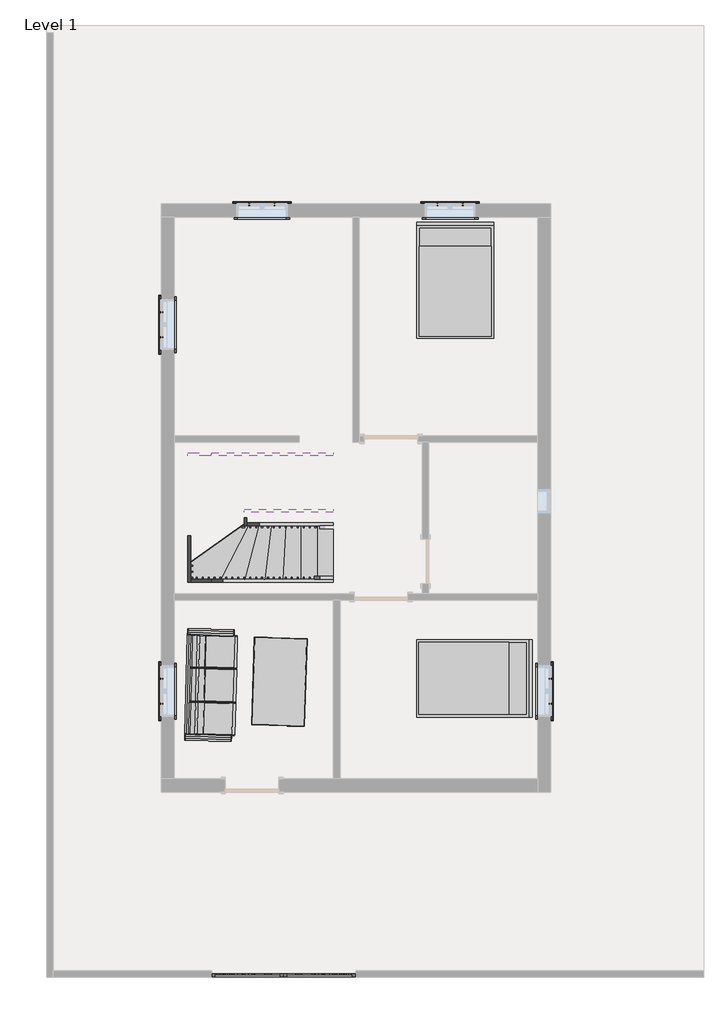
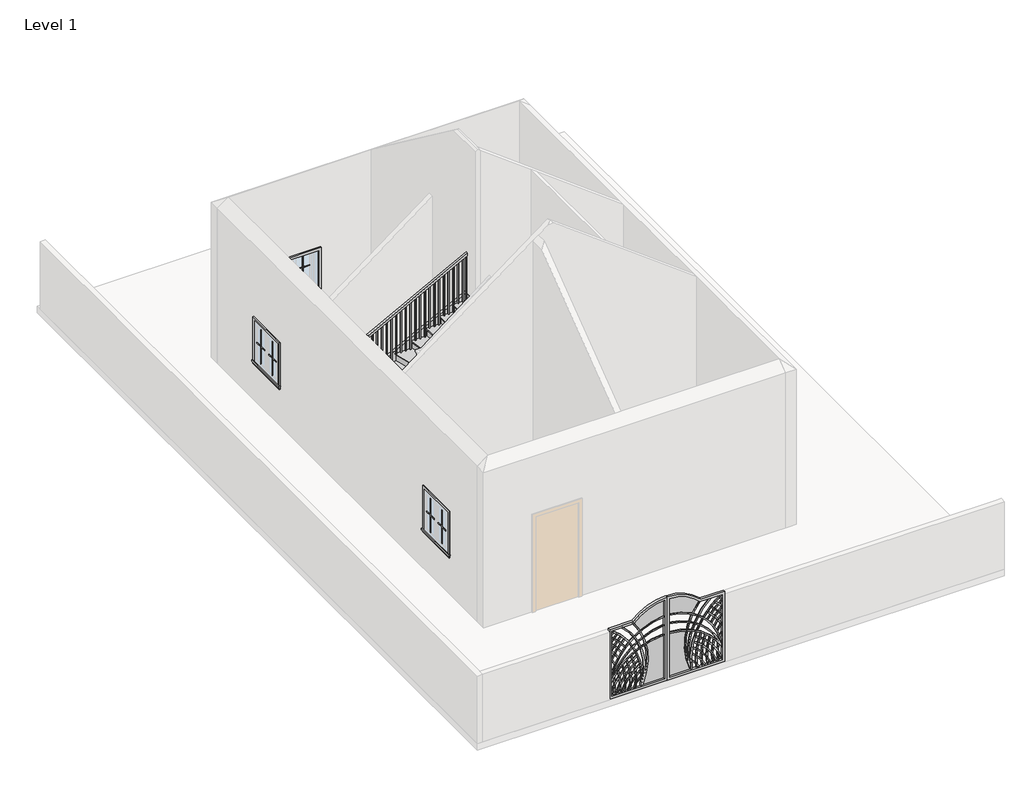
# One storey, part 2 of 2: 21 proxies, 8 members, 4 furniture elements, 1 railing, 1 stair flight.
"""IFC4 building model written with IfcOpenShell, lengths in millimetres."""

from ifc_helpers import new_model, si_unit, frame, origin, place, context, project, spatial, polyline, outline, extrude, faceted_brep, transform, mapped, element, save
from components import generic_models_6bc30956, muntin_pattern_2x2_muntin_pattern_2x2_b3fe6957, muntin_pattern_2x2_muntin_pattern_2x2_3e0ecaf2, trim_window_exterior_flat_with_sill_41619996, trim_window_interior_flat_picture_frame_51c85655, furniture_2fc85b74, furniture_29a9adb8, furniture_57072a26, bed_17739_bed_17739_15c61121, dining_table_14755_dining_table_14755_d89cb775, stair_flight_6e6a5ea5

model = new_model("IFC4")

# Units and contexts
model_context = context("Model", 3, world=origin())
ifc_project = project(units=[si_unit("LENGTHUNIT", "METRE", prefix="MILLI")], contexts=[model_context])

# Site, building, storey
site = spatial("IfcSite", under=ifc_project)
building = spatial("IfcBuilding", under=site)
storey = spatial("IfcBuildingStorey", under=building, Name="Level 1", Elevation=0.0)

# Proxies
placement = place(None, origin())
generic_models_shape = generic_models_6bc30956(model_context)
element("IfcBuildingElementProxy", 1, Name="Generic Models", at=placement, inside=storey, context=model_context, shape_type="MappedRepresentation", body=[
    mapped(generic_models_shape, transform((-2517.3949167, -8004.7025057, 0.0), x_axis=(1.0, 0.0, 0.0), y_axis=(0.0, 1.0, 0.0), z_axis=(0.0, 0.0, 1.0))),
])
muntin_pattern_2x2_muntin_pattern_2x2_shape = muntin_pattern_2x2_muntin_pattern_2x2_b3fe6957(model_context)
element("IfcBuildingElementProxy", 2, Name="Muntin Pattern_2x2 : Muntin Pattern_2x2", ObjectType="Muntin Pattern_2x2 : Muntin Pattern_2x2", at=placement, inside=storey, context=model_context, shape_type="MappedRepresentation", body=[
    mapped(muntin_pattern_2x2_muntin_pattern_2x2_shape, transform((-3096.8324167, 5150.2179147, 984.25), x_axis=(1.0, 0.0, 0.0), y_axis=(0.0, 1.0, 0.0), z_axis=(0.0, 0.0, 1.0))),
])
element("IfcBuildingElementProxy", 3, Name="Muntin Pattern_2x2 : Muntin Pattern_2x2", ObjectType="Muntin Pattern_2x2 : Muntin Pattern_2x2", at=placement, inside=storey, context=model_context, shape_type="MappedRepresentation", body=[
    mapped(muntin_pattern_2x2_muntin_pattern_2x2_shape, transform((122.6175833, 5150.2179147, 984.25), x_axis=(1.0, 0.0, 0.0), y_axis=(0.0, 1.0, 0.0), z_axis=(0.0, 0.0, 1.0))),
])
element("IfcBuildingElementProxy", 4, Name="Muntin Pattern_2x2 : Muntin Pattern_2x2", ObjectType="Muntin Pattern_2x2 : Muntin Pattern_2x2", at=placement, inside=storey, context=model_context, shape_type="MappedRepresentation", body=[
    mapped(muntin_pattern_2x2_muntin_pattern_2x2_shape, transform((2051.4300833, -2960.3195853, 984.25), x_axis=(0.0, -1.0, 0.0), y_axis=(1.0, 0.0, 0.0), z_axis=(0.0, 0.0, 1.0))),
])
element("IfcBuildingElementProxy", 5, Name="Muntin Pattern_2x2 : Muntin Pattern_2x2", ObjectType="Muntin Pattern_2x2 : Muntin Pattern_2x2", at=placement, inside=storey, context=model_context, shape_type="MappedRepresentation", body=[
    mapped(muntin_pattern_2x2_muntin_pattern_2x2_shape, transform((-4597.0199167, 2878.5054147, 984.25), x_axis=(0.0, 1.0, 0.0), y_axis=(-1.0, 0.0, 0.0), z_axis=(0.0, 0.0, 1.0))),
])
element("IfcBuildingElementProxy", 6, Name="Muntin Pattern_2x2 : Muntin Pattern_2x2", ObjectType="Muntin Pattern_2x2 : Muntin Pattern_2x2", at=placement, inside=storey, context=model_context, shape_type="MappedRepresentation", body=[
    mapped(muntin_pattern_2x2_muntin_pattern_2x2_shape, transform((-4597.0199167, -3388.9445853, 984.25), x_axis=(0.0, 1.0, 0.0), y_axis=(-1.0, 0.0, 0.0), z_axis=(0.0, 0.0, 1.0))),
])
muntin_pattern_2x2_muntin_pattern_2x2_2_shape = muntin_pattern_2x2_muntin_pattern_2x2_3e0ecaf2(model_context)
element("IfcBuildingElementProxy", 7, Name="Muntin Pattern_2x2 : Muntin Pattern_2x2", ObjectType="Muntin Pattern_2x2 : Muntin Pattern_2x2", at=placement, inside=storey, context=model_context, shape_type="MappedRepresentation", body=[
    mapped(muntin_pattern_2x2_muntin_pattern_2x2_2_shape, transform((-2668.2074167, 5150.2179147, 984.25), x_axis=(-1.0, 0.0, 0.0), y_axis=(0.0, -1.0, 0.0), z_axis=(0.0, 0.0, 1.0))),
])
element("IfcBuildingElementProxy", 8, Name="Muntin Pattern_2x2 : Muntin Pattern_2x2", ObjectType="Muntin Pattern_2x2 : Muntin Pattern_2x2", at=placement, inside=storey, context=model_context, shape_type="MappedRepresentation", body=[
    mapped(muntin_pattern_2x2_muntin_pattern_2x2_2_shape, transform((551.2425833, 5150.2179147, 984.25), x_axis=(-1.0, 0.0, 0.0), y_axis=(0.0, -1.0, 0.0), z_axis=(0.0, 0.0, 1.0))),
])
element("IfcBuildingElementProxy", 9, Name="Muntin Pattern_2x2 : Muntin Pattern_2x2", ObjectType="Muntin Pattern_2x2 : Muntin Pattern_2x2", at=placement, inside=storey, context=model_context, shape_type="MappedRepresentation", body=[
    mapped(muntin_pattern_2x2_muntin_pattern_2x2_2_shape, transform((2051.4300833, -3388.9445853, 984.25), x_axis=(0.0, 1.0, 0.0), y_axis=(-1.0, 0.0, 0.0), z_axis=(0.0, 0.0, 1.0))),
])
element("IfcBuildingElementProxy", 10, Name="Muntin Pattern_2x2 : Muntin Pattern_2x2", ObjectType="Muntin Pattern_2x2 : Muntin Pattern_2x2", at=placement, inside=storey, context=model_context, shape_type="MappedRepresentation", body=[
    mapped(muntin_pattern_2x2_muntin_pattern_2x2_2_shape, transform((-4597.0199167, 3307.1304147, 984.25), x_axis=(0.0, -1.0, 0.0), y_axis=(1.0, 0.0, 0.0), z_axis=(0.0, 0.0, 1.0))),
])
element("IfcBuildingElementProxy", 11, Name="Muntin Pattern_2x2 : Muntin Pattern_2x2", ObjectType="Muntin Pattern_2x2 : Muntin Pattern_2x2", at=placement, inside=storey, context=model_context, shape_type="MappedRepresentation", body=[
    mapped(muntin_pattern_2x2_muntin_pattern_2x2_2_shape, transform((-4597.0199167, -2960.3195853, 984.25), x_axis=(0.0, -1.0, 0.0), y_axis=(1.0, 0.0, 0.0), z_axis=(0.0, 0.0, 1.0))),
])
trim_window_exterior_flat_with_sill_shape = trim_window_exterior_flat_with_sill_41619996(model_context)
element("IfcBuildingElementProxy", 12, Name="Trim-Window-Exterior-Flat : with Sill", ObjectType="Trim-Window-Exterior-Flat : with Sill", at=placement, inside=storey, context=model_context, shape_type="MappedRepresentation", body=[
    mapped(trim_window_exterior_flat_with_sill_shape, transform((-2882.5199167, 5159.7429147, 1828.8), x_axis=(-1.0, 0.0, 0.0), y_axis=(0.0, 0.0, 1.0), z_axis=(0.0, 1.0, 0.0))),
])
element("IfcBuildingElementProxy", 13, Name="Trim-Window-Exterior-Flat : with Sill", ObjectType="Trim-Window-Exterior-Flat : with Sill", at=placement, inside=storey, context=model_context, shape_type="MappedRepresentation", body=[
    mapped(trim_window_exterior_flat_with_sill_shape, transform((336.9300833, 5159.7429147, 1828.8), x_axis=(-1.0, 0.0, 0.0), y_axis=(0.0, 0.0, 1.0), z_axis=(0.0, 1.0, 0.0))),
])
element("IfcBuildingElementProxy", 14, Name="Trim-Window-Exterior-Flat : with Sill", ObjectType="Trim-Window-Exterior-Flat : with Sill", at=placement, inside=storey, context=model_context, shape_type="MappedRepresentation", body=[
    mapped(trim_window_exterior_flat_with_sill_shape, transform((2060.9550833, -3174.6320853, 1828.8), x_axis=(0.0, 1.0, 0.0), y_axis=(0.0, 0.0, 1.0), z_axis=(1.0, 0.0, 0.0))),
])
element("IfcBuildingElementProxy", 15, Name="Trim-Window-Exterior-Flat : with Sill", ObjectType="Trim-Window-Exterior-Flat : with Sill", at=placement, inside=storey, context=model_context, shape_type="MappedRepresentation", body=[
    mapped(trim_window_exterior_flat_with_sill_shape, transform((-4606.5449167, 3092.8179147, 1828.8), x_axis=(0.0, -1.0, 0.0), y_axis=(0.0, 0.0, 1.0), z_axis=(-1.0, 0.0, 0.0))),
])
element("IfcBuildingElementProxy", 16, Name="Trim-Window-Exterior-Flat : with Sill", ObjectType="Trim-Window-Exterior-Flat : with Sill", at=placement, inside=storey, context=model_context, shape_type="MappedRepresentation", body=[
    mapped(trim_window_exterior_flat_with_sill_shape, transform((-4606.5449167, -3174.6320853, 1828.8), x_axis=(0.0, -1.0, 0.0), y_axis=(0.0, 0.0, 1.0), z_axis=(-1.0, 0.0, 0.0))),
])
trim_window_interior_flat_picture_frame_shape = trim_window_interior_flat_picture_frame_51c85655(model_context)
element("IfcBuildingElementProxy", 17, Name="Trim-Window-Interior-Flat : Picture Frame", ObjectType="Trim-Window-Interior-Flat : Picture Frame", at=placement, inside=storey, context=model_context, shape_type="MappedRepresentation", body=[
    mapped(trim_window_interior_flat_picture_frame_shape, transform((-2882.5199167, 4931.1429147, 1828.8), x_axis=(1.0, 0.0, 0.0), y_axis=(0.0, 0.0, 1.0), z_axis=(0.0, -1.0, 0.0))),
])
element("IfcBuildingElementProxy", 18, Name="Trim-Window-Interior-Flat : Picture Frame", ObjectType="Trim-Window-Interior-Flat : Picture Frame", at=placement, inside=storey, context=model_context, shape_type="MappedRepresentation", body=[
    mapped(trim_window_interior_flat_picture_frame_shape, transform((336.9300833, 4931.1429147, 1828.8), x_axis=(1.0, 0.0, 0.0), y_axis=(0.0, 0.0, 1.0), z_axis=(0.0, -1.0, 0.0))),
])
element("IfcBuildingElementProxy", 19, Name="Trim-Window-Interior-Flat : Picture Frame", ObjectType="Trim-Window-Interior-Flat : Picture Frame", at=placement, inside=storey, context=model_context, shape_type="MappedRepresentation", body=[
    mapped(trim_window_interior_flat_picture_frame_shape, transform((1832.3550833, -3174.6320853, 1828.8), x_axis=(0.0, -1.0, 0.0), y_axis=(0.0, 0.0, 1.0), z_axis=(-1.0, 0.0, 0.0))),
])
element("IfcBuildingElementProxy", 20, Name="Trim-Window-Interior-Flat : Picture Frame", ObjectType="Trim-Window-Interior-Flat : Picture Frame", at=placement, inside=storey, context=model_context, shape_type="MappedRepresentation", body=[
    mapped(trim_window_interior_flat_picture_frame_shape, transform((-4377.9449167, 3092.8179147, 1828.8), x_axis=(0.0, 1.0, 0.0), y_axis=(0.0, 0.0, 1.0), z_axis=(1.0, 0.0, 0.0))),
])
element("IfcBuildingElementProxy", 21, Name="Trim-Window-Interior-Flat : Picture Frame", ObjectType="Trim-Window-Interior-Flat : Picture Frame", at=placement, inside=storey, context=model_context, shape_type="MappedRepresentation", body=[
    mapped(trim_window_interior_flat_picture_frame_shape, transform((-4377.9449167, -3174.6320853, 1828.8), x_axis=(0.0, 1.0, 0.0), y_axis=(0.0, 0.0, 1.0), z_axis=(1.0, 0.0, 0.0))),
])

# Furniture
furniture_shape = furniture_2fc85b74(model_context)
furniture_2_shape = furniture_29a9adb8(model_context)
furniture_3_shape = furniture_57072a26(model_context)
element("IfcFurniture", 22, at=placement, inside=storey, context=model_context, shape_type="MappedRepresentation", body=[
    mapped(furniture_shape, transform((-3377.5302414, -3078.4784971, 0.0), x_axis=(0.026303757153397337, 0.9996539963205345, 0.0), y_axis=(-0.9996539963205345, 0.026303757153397337, 0.0), z_axis=(0.0, 0.0, 1.0))),
    mapped(furniture_2_shape, transform((-3377.5302414, -3078.4784971, 0.0), x_axis=(0.026303757153397337, 0.9996539963205345, 0.0), y_axis=(-0.9996539963205345, 0.026303757153397337, 0.0), z_axis=(0.0, 0.0, 1.0))),
    mapped(furniture_3_shape, transform((-3377.5302414, -3078.4784971, 0.0), x_axis=(0.026303757153397337, 0.9996539963205345, 0.0), y_axis=(-0.9996539963205345, 0.026303757153397337, 0.0), z_axis=(0.0, 0.0, 1.0))),
])
bed_17739_bed_17739_shape = bed_17739_bed_17739_15c61121(model_context)
element("IfcFurniture", 23, ObjectType="Bed_17739 : Bed_17739", at=placement, inside=storey, context=model_context, shape_type="MappedRepresentation", body=[
    mapped(bed_17739_bed_17739_shape, transform((422.6550833, 3826.2429147, 0.0), x_axis=(1.0, 0.0, 0.0), y_axis=(0.0, 1.0, 0.0), z_axis=(0.0, 0.0, 1.0))),
])
element("IfcFurniture", 24, ObjectType="Bed_17739 : Bed_17739", at=placement, inside=storey, context=model_context, shape_type="MappedRepresentation", body=[
    mapped(bed_17739_bed_17739_shape, transform((727.4550833, -2955.5570853, 0.0), x_axis=(0.0, -1.0, 0.0), y_axis=(1.0, 0.0, 0.0), z_axis=(0.0, 0.0, 1.0))),
])
dining_table_14755_dining_table_14755_shape = dining_table_14755_dining_table_14755_d89cb775(model_context)
element("IfcFurniture", 25, ObjectType="Dining_table_14755 : Dining_table_14755", at=placement, inside=storey, context=model_context, shape_type="MappedRepresentation", body=[
    mapped(dining_table_14755_dining_table_14755_shape, transform((-2158.9663672, -3776.6607291, 0.0), x_axis=(0.0325552683465733, 0.9994699367679264, 0.0), y_axis=(-0.9994699367679264, 0.0325552683465733, 0.0), z_axis=(0.0, 0.0, 1.0))),
])

# Members
element("IfcMember", 26, ObjectType="Stringer - 2\" Width", at=placement, inside=storey, context=model_context, shape_type="SweptSolid", body=[
    extrude(outline(polyline([(0.0, -1660.1449167), (229.639954, -1660.1449167), (1305.3956453, -3747.5621084), (962.500629, -3747.5621084), (0.0, -1879.9072342), (0.0, -1660.1449167)])), frame((0.0, -1310.9070853, 0.0), z_axis=(0.0, 1.0, 0.0), x_axis=(0.0, 0.0, 1.0)), (0.0, 0.0, 1.0), 50.8),
])
element("IfcMember", 27, ObjectType="Stringer - 2\" Width", at=placement, inside=storey, context=model_context, shape_type="SweptSolid", body=[
    extrude(outline(polyline([(-3747.5621084, -1260.1070853), (-3747.5621084, -1310.9070853), (-4102.2766085, -1310.9070853), (-4102.2766085, -1260.1070853), (-3747.5621084, -1260.1070853)])), frame((0.0, 0.0, 962.500629), z_axis=(0.0, 0.0, 1.0), x_axis=(1.0, 0.0, 0.0)), (0.0, 0.0, 1.0), 342.8950162),
])
element("IfcMember", 28, ObjectType="Stringer - 2\" Width", at=placement, inside=storey, context=model_context, shape_type="SweptSolid", body=[
    extrude(outline(polyline([(-1310.9070853, 1000.5956453), (-1310.9070853, 1289.0952212), (811.1127974, 1969.9972697), (848.0929147, 1969.9972697), (848.0929147, 1638.9682298), (-1141.3846024, 1000.5956453), (-1310.9070853, 1000.5956453)])), frame((-4153.0766085, 0.0, 0.0), z_axis=(1.0, 0.0, 0.0), x_axis=(0.0, 1.0, 0.0)), (0.0, 0.0, 1.0), 50.8),
])
element("IfcMember", 29, ObjectType="Stringer - 2\" Width", at=placement, inside=storey, context=model_context, shape_type="SweptSolid", body=[
    extrude(outline(polyline([(-4153.0766085, 848.0929147), (-4153.0766085, 898.8929147), (-3747.5621084, 898.8929147), (-3747.5621084, 848.0929147), (-4153.0766085, 848.0929147)])), frame((0.0, 0.0, 1649.8904473), z_axis=(0.0, 0.0, 1.0), x_axis=(1.0, 0.0, 0.0)), (0.0, 0.0, 1.0), 320.1068224),
])
element("IfcMember", 30, ObjectType="Stringer - 2\" Width", at=placement, inside=storey, context=model_context, shape_type="SweptSolid", body=[
    extrude(outline(polyline([(1969.9972697, -3747.5621084), (1649.8904473, -3747.5621084), (2725.6461385, -1660.1449167), (3045.7529609, -1660.1449167), (1969.9972697, -3747.5621084)])), frame((0.0, 848.0929147, 0.0), z_axis=(0.0, 1.0, 0.0), x_axis=(0.0, 0.0, 1.0)), (0.0, 0.0, 1.0), 50.8),
])
element("IfcMember", 31, ObjectType="Stringer - 2\" Width", at=placement, inside=storey, context=model_context, shape_type="SweptSolid", body=[
    extrude(outline(polyline([(0.0, -1660.1449167), (176.1764461, -1660.1449167), (1380.418648, -3137.0766085), (987.1410923, -3137.0766085), (0.0, -1926.4065612), (0.0, -1660.1449167)])), frame((0.0, -345.7070853, 0.0), z_axis=(0.0, 1.0, 0.0), x_axis=(0.0, 0.0, 1.0)), (0.0, 0.0, 1.0), 50.8),
])
element("IfcMember", 32, ObjectType="Stringer - 2\" Width", at=placement, inside=storey, context=model_context, shape_type="SweptSolid", body=[
    extrude(outline(polyline([(-345.7070853, 1028.5617647), (-345.7070853, 1573.2682978), (-139.0699679, 1926.1409689), (-117.1070853, 1926.1409689), (-117.1070853, 1360.465107), (-311.464868, 1028.5617647), (-345.7070853, 1028.5617647)])), frame((-3187.8766085, 0.0, 0.0), z_axis=(1.0, 0.0, 0.0), x_axis=(0.0, 1.0, 0.0)), (0.0, 0.0, 1.0), 50.8),
])
element("IfcMember", 33, ObjectType="Stringer - 2\" Width", at=placement, inside=storey, context=model_context, shape_type="SweptSolid", body=[
    extrude(outline(polyline([(1926.1409689, -3187.8766085), (1532.8634131, -3187.8766085), (2778.5262875, -1660.1449167), (3171.8038432, -1660.1449167), (1926.1409689, -3187.8766085)])), frame((0.0, -117.1070853, 0.0), z_axis=(0.0, 1.0, 0.0), x_axis=(0.0, 0.0, 1.0)), (0.0, 0.0, 1.0), 50.8),
])

# Railing
element("IfcRailing", 34, ObjectType="Handrail - Rectangular", at=placement, inside=storey, context=model_context, shape_type="SolidModel", body=[
    faceted_brep([(-1660.1449167, -1260.1070853, 1083.7333333), (-1660.1449167, -1260.1070853, 1026.2742652), (-1660.1449167, -1209.3070853, 1026.2742652), (-1660.1449167, -1209.3070853, 1083.7333333), (-3917.8699787, -1260.1070853, 2277.0239201), (-3930.4690433, -1260.1070853, 2226.2239201), (-3930.4690433, -1209.3070853, 2226.2239201), (-3917.8699787, -1209.3070853, 2277.0239201), (-4102.2766085, -1260.1070853, 2277.0239201), (-4102.2766085, -1260.1070853, 2226.2239201), (-4051.4766085, -1209.3070853, 2226.2239201), (-4051.4766085, -1209.3070853, 2277.0239201), (-4102.2766085, -972.7952032, 2277.0239201), (-4102.2766085, -964.8446271, 2226.2239201), (-4051.4766085, -964.8446271, 2226.2239201), (-4051.4766085, -972.7952032, 2277.0239201), (-4102.2766085, 560.7810325, 2769.1094132), (-4102.2766085, 568.7316087, 2718.3094132), (-4051.4766085, 568.7316087, 2718.3094132), (-4051.4766085, 560.7810325, 2769.1094132), (-4102.2766085, 848.0929147, 2769.1094132), (-4102.2766085, 848.0929147, 2718.3094132), (-4051.4766085, 797.2929147, 2718.3094132), (-4051.4766085, 797.2929147, 2769.1094132), (-3917.8699787, 848.0929147, 2769.1094132), (-3905.2709142, 848.0929147, 2718.3094132), (-3905.2709142, 797.2929147, 2718.3094132), (-3917.8699787, 797.2929147, 2769.1094132), (-1660.1449167, 848.0929147, 3962.4), (-1660.1449167, 797.2929147, 3962.4), (-1660.1449167, 797.2929147, 3904.9409318), (-1660.1449167, 848.0929147, 3904.9409318)], [[[0, 1, 2, 3]], [[1, 0, 4, 5]], [[2, 1, 5, 6]], [[3, 2, 6, 7]], [[0, 3, 7, 4]], [[5, 4, 8, 9]], [[6, 5, 9, 10]], [[7, 6, 10, 11]], [[4, 7, 11, 8]], [[9, 8, 12, 13]], [[10, 9, 13, 14]], [[11, 10, 14, 15]], [[8, 11, 15, 12]], [[13, 12, 16, 17]], [[14, 13, 17, 18]], [[15, 14, 18, 19]], [[12, 15, 19, 16]], [[17, 16, 20, 21]], [[18, 17, 21, 22]], [[19, 18, 22, 23]], [[16, 19, 23, 20]], [[21, 20, 24, 25]], [[22, 21, 25, 26]], [[23, 22, 26, 27]], [[20, 23, 27, 24]], [[28, 29, 30, 31]], [[25, 24, 28, 31]], [[26, 25, 31, 30]], [[27, 26, 30, 29]], [[24, 27, 29, 28]]]),
    extrude(outline(polyline([(3857.6597858, -1749.6016085), (2878.6666667, -1749.6016085), (2878.6666667, -1730.5516085), (3867.7284102, -1730.5516085), (3857.6597858, -1749.6016085)])), frame((0.0, 813.1679147, 0.0), z_axis=(0.0, 1.0, 0.0), x_axis=(0.0, 0.0, 1.0)), (0.0, 0.0, 1.0), 19.05),
    extrude(outline(polyline([(3803.9604556, -1851.2016085), (2878.6666667, -1851.2016085), (2878.6666667, -1832.1516085), (3814.02908, -1832.1516085), (3803.9604556, -1851.2016085)])), frame((0.0, 813.1679147, 0.0), z_axis=(0.0, 1.0, 0.0), x_axis=(0.0, 0.0, 1.0)), (0.0, 0.0, 1.0), 19.05),
    extrude(outline(polyline([(3750.2611254, -1952.8016085), (2709.3333333, -1952.8016085), (2709.3333333, -1933.7516085), (3760.3297498, -1933.7516085), (3750.2611254, -1952.8016085)])), frame((0.0, 813.1679147, 0.0), z_axis=(0.0, 1.0, 0.0), x_axis=(0.0, 0.0, 1.0)), (0.0, 0.0, 1.0), 19.05),
    extrude(outline(polyline([(3696.5617952, -2054.4016085), (2709.3333333, -2054.4016085), (2709.3333333, -2035.3516085), (3706.6304196, -2035.3516085), (3696.5617952, -2054.4016085)])), frame((0.0, 813.1679147, 0.0), z_axis=(0.0, 1.0, 0.0), x_axis=(0.0, 0.0, 1.0)), (0.0, 0.0, 1.0), 19.05),
    extrude(outline(polyline([(3642.862465, -2156.0016085), (2709.3333333, -2156.0016085), (2709.3333333, -2136.9516085), (3652.9310894, -2136.9516085), (3642.862465, -2156.0016085)])), frame((0.0, 813.1679147, 0.0), z_axis=(0.0, 1.0, 0.0), x_axis=(0.0, 0.0, 1.0)), (0.0, 0.0, 1.0), 19.05),
    extrude(outline(polyline([(3589.1631348, -2257.6016085), (2540.0, -2257.6016085), (2540.0, -2238.5516085), (3599.2317592, -2238.5516085), (3589.1631348, -2257.6016085)])), frame((0.0, 813.1679147, 0.0), z_axis=(0.0, 1.0, 0.0), x_axis=(0.0, 0.0, 1.0)), (0.0, 0.0, 1.0), 19.05),
    extrude(outline(polyline([(3535.4638046, -2359.2016085), (2540.0, -2359.2016085), (2540.0, -2340.1516085), (3545.532429, -2340.1516085), (3535.4638046, -2359.2016085)])), frame((0.0, 813.1679147, 0.0), z_axis=(0.0, 1.0, 0.0), x_axis=(0.0, 0.0, 1.0)), (0.0, 0.0, 1.0), 19.05),
    extrude(outline(polyline([(3481.7644744, -2460.8016085), (2540.0, -2460.8016085), (2540.0, -2441.7516085), (3491.8330988, -2441.7516085), (3481.7644744, -2460.8016085)])), frame((0.0, 813.1679147, 0.0), z_axis=(0.0, 1.0, 0.0), x_axis=(0.0, 0.0, 1.0)), (0.0, 0.0, 1.0), 19.05),
    extrude(outline(polyline([(3428.0651442, -2562.4016085), (2370.6666667, -2562.4016085), (2370.6666667, -2543.3516085), (3438.1337686, -2543.3516085), (3428.0651442, -2562.4016085)])), frame((0.0, 813.1679147, 0.0), z_axis=(0.0, 1.0, 0.0), x_axis=(0.0, 0.0, 1.0)), (0.0, 0.0, 1.0), 19.05),
    extrude(outline(polyline([(3374.365814, -2664.0016085), (2370.6666667, -2664.0016085), (2370.6666667, -2644.9516085), (3384.4344384, -2644.9516085), (3374.365814, -2664.0016085)])), frame((0.0, 813.1679147, 0.0), z_axis=(0.0, 1.0, 0.0), x_axis=(0.0, 0.0, 1.0)), (0.0, 0.0, 1.0), 19.05),
    extrude(outline(polyline([(3320.6664838, -2765.6016085), (2370.6666667, -2765.6016085), (2370.6666667, -2746.5516085), (3330.7351082, -2746.5516085), (3320.6664838, -2765.6016085)])), frame((0.0, 813.1679147, 0.0), z_axis=(0.0, 1.0, 0.0), x_axis=(0.0, 0.0, 1.0)), (0.0, 0.0, 1.0), 19.05),
    extrude(outline(polyline([(3266.9671536, -2867.2016085), (2201.3333333, -2867.2016085), (2201.3333333, -2848.1516085), (3277.035778, -2848.1516085), (3266.9671536, -2867.2016085)])), frame((0.0, 813.1679147, 0.0), z_axis=(0.0, 1.0, 0.0), x_axis=(0.0, 0.0, 1.0)), (0.0, 0.0, 1.0), 19.05),
    extrude(outline(polyline([(3213.2678234, -2968.8016085), (2201.3333333, -2968.8016085), (2201.3333333, -2949.7516085), (3223.3364478, -2949.7516085), (3213.2678234, -2968.8016085)])), frame((0.0, 813.1679147, 0.0), z_axis=(0.0, 1.0, 0.0), x_axis=(0.0, 0.0, 1.0)), (0.0, 0.0, 1.0), 19.05),
    extrude(outline(polyline([(3159.5684932, -3070.4016085), (2201.3333333, -3070.4016085), (2201.3333333, -3051.3516085), (3169.6371176, -3051.3516085), (3159.5684932, -3070.4016085)])), frame((0.0, 813.1679147, 0.0), z_axis=(0.0, 1.0, 0.0), x_axis=(0.0, 0.0, 1.0)), (0.0, 0.0, 1.0), 19.05),
    extrude(outline(polyline([(3105.869163, -3172.0016085), (2201.3333333, -3172.0016085), (2201.3333333, -3152.9516085), (3115.9377874, -3152.9516085), (3105.869163, -3172.0016085)])), frame((0.0, 813.1679147, 0.0), z_axis=(0.0, 1.0, 0.0), x_axis=(0.0, 0.0, 1.0)), (0.0, 0.0, 1.0), 19.05),
    extrude(outline(polyline([(3052.1698328, -3273.6016085), (2032.0, -3273.6016085), (2032.0, -3254.5516085), (3062.2384572, -3254.5516085), (3052.1698328, -3273.6016085)])), frame((0.0, 813.1679147, 0.0), z_axis=(0.0, 1.0, 0.0), x_axis=(0.0, 0.0, 1.0)), (0.0, 0.0, 1.0), 19.05),
    extrude(outline(polyline([(2998.4705026, -3375.2016085), (2032.0, -3375.2016085), (2032.0, -3356.1516085), (3008.539127, -3356.1516085), (2998.4705026, -3375.2016085)])), frame((0.0, 813.1679147, 0.0), z_axis=(0.0, 1.0, 0.0), x_axis=(0.0, 0.0, 1.0)), (0.0, 0.0, 1.0), 19.05),
    extrude(outline(polyline([(2944.7711724, -3476.8016085), (2032.0, -3476.8016085), (2032.0, -3457.7516085), (2954.8397968, -3457.7516085), (2944.7711724, -3476.8016085)])), frame((0.0, 813.1679147, 0.0), z_axis=(0.0, 1.0, 0.0), x_axis=(0.0, 0.0, 1.0)), (0.0, 0.0, 1.0), 19.05),
    extrude(outline(polyline([(2891.0718422, -3578.4016085), (2032.0, -3578.4016085), (2032.0, -3559.3516085), (2901.1404666, -3559.3516085), (2891.0718422, -3578.4016085)])), frame((0.0, 813.1679147, 0.0), z_axis=(0.0, 1.0, 0.0), x_axis=(0.0, 0.0, 1.0)), (0.0, 0.0, 1.0), 19.05),
    extrude(outline(polyline([(2837.372512, -3680.0016085), (1862.6666667, -3680.0016085), (1862.6666667, -3660.9516085), (2847.4411364, -3660.9516085), (2837.372512, -3680.0016085)])), frame((0.0, 813.1679147, 0.0), z_axis=(0.0, 1.0, 0.0), x_axis=(0.0, 0.0, 1.0)), (0.0, 0.0, 1.0), 19.05),
    extrude(outline(polyline([(2783.6731818, -3781.6016085), (1862.6666667, -3781.6016085), (1862.6666667, -3762.5516085), (2793.7418062, -3762.5516085), (2783.6731818, -3781.6016085)])), frame((0.0, 813.1679147, 0.0), z_axis=(0.0, 1.0, 0.0), x_axis=(0.0, 0.0, 1.0)), (0.0, 0.0, 1.0), 19.05),
    extrude(outline(polyline([(2729.9738516, -3883.2016085), (1862.6666667, -3883.2016085), (1862.6666667, -3864.1516085), (2740.042476, -3864.1516085), (2729.9738516, -3883.2016085)])), frame((0.0, 813.1679147, 0.0), z_axis=(0.0, 1.0, 0.0), x_axis=(0.0, 0.0, 1.0)), (0.0, 0.0, 1.0), 19.05),
    extrude(outline(polyline([(-3984.8016085, 832.2179147), (-3965.7516085, 832.2179147), (-3965.7516085, 813.1679147), (-3984.8016085, 813.1679147), (-3984.8016085, 832.2179147)])), frame((0.0, 0.0, 1862.6666667), z_axis=(0.0, 0.0, 1.0), x_axis=(1.0, 0.0, 0.0)), (0.0, 0.0, 1.0), 855.6427466),
    extrude(outline(polyline([(-4086.4016085, 787.7679147), (-4086.4016085, 806.8179147), (-4067.3516085, 806.8179147), (-4067.3516085, 787.7679147), (-4086.4016085, 787.7679147)])), frame((0.0, 0.0, 1862.6666667), z_axis=(0.0, 0.0, 1.0), x_axis=(1.0, 0.0, 0.0)), (0.0, 0.0, 1.0), 855.6427466),
    extrude(outline(polyline([(-4086.4016085, 686.1679147), (-4086.4016085, 705.2179147), (-4067.3516085, 705.2179147), (-4067.3516085, 686.1679147), (-4086.4016085, 686.1679147)])), frame((0.0, 0.0, 1862.6666667), z_axis=(0.0, 0.0, 1.0), x_axis=(1.0, 0.0, 0.0)), (0.0, 0.0, 1.0), 855.6427466),
    extrude(outline(polyline([(-4086.4016085, 584.5679147), (-4086.4016085, 603.6179147), (-4067.3516085, 603.6179147), (-4067.3516085, 584.5679147), (-4086.4016085, 584.5679147)])), frame((0.0, 0.0, 1862.6666667), z_axis=(0.0, 0.0, 1.0), x_axis=(1.0, 0.0, 0.0)), (0.0, 0.0, 1.0), 855.6427466),
    extrude(outline(polyline([(502.0179147, 2696.9026907), (502.0179147, 1693.3333333), (482.9679147, 1693.3333333), (482.9679147, 2690.7900316), (502.0179147, 2696.9026907)])), frame((-4086.4016085, 0.0, 0.0), z_axis=(1.0, 0.0, 0.0), x_axis=(0.0, 1.0, 0.0)), (0.0, 0.0, 1.0), 19.05),
    extrude(outline(polyline([(400.4179147, 2664.3018425), (400.4179147, 1693.3333333), (381.3679147, 1693.3333333), (381.3679147, 2658.1891834), (400.4179147, 2664.3018425)])), frame((-4086.4016085, 0.0, 0.0), z_axis=(1.0, 0.0, 0.0), x_axis=(0.0, 1.0, 0.0)), (0.0, 0.0, 1.0), 19.05),
    extrude(outline(polyline([(298.8179147, 2631.7009942), (298.8179147, 1693.3333333), (279.7679147, 1693.3333333), (279.7679147, 2625.5883352), (298.8179147, 2631.7009942)])), frame((-4086.4016085, 0.0, 0.0), z_axis=(1.0, 0.0, 0.0), x_axis=(0.0, 1.0, 0.0)), (0.0, 0.0, 1.0), 19.05),
    extrude(outline(polyline([(197.2179147, 2599.100146), (197.2179147, 1693.3333333), (178.1679147, 1693.3333333), (178.1679147, 2592.987487), (197.2179147, 2599.100146)])), frame((-4086.4016085, 0.0, 0.0), z_axis=(1.0, 0.0, 0.0), x_axis=(0.0, 1.0, 0.0)), (0.0, 0.0, 1.0), 19.05),
    extrude(outline(polyline([(95.6179147, 2566.4992978), (95.6179147, 1693.3333333), (76.5679147, 1693.3333333), (76.5679147, 2560.3866387), (95.6179147, 2566.4992978)])), frame((-4086.4016085, 0.0, 0.0), z_axis=(1.0, 0.0, 0.0), x_axis=(0.0, 1.0, 0.0)), (0.0, 0.0, 1.0), 19.05),
    extrude(outline(polyline([(-5.9820853, 2533.8984495), (-5.9820853, 1524.0), (-25.0320853, 1524.0), (-25.0320853, 2527.7857905), (-5.9820853, 2533.8984495)])), frame((-4086.4016085, 0.0, 0.0), z_axis=(1.0, 0.0, 0.0), x_axis=(0.0, 1.0, 0.0)), (0.0, 0.0, 1.0), 19.05),
    extrude(outline(polyline([(-107.5820853, 2501.2976013), (-107.5820853, 1524.0), (-126.6320853, 1524.0), (-126.6320853, 2495.1849423), (-107.5820853, 2501.2976013)])), frame((-4086.4016085, 0.0, 0.0), z_axis=(1.0, 0.0, 0.0), x_axis=(0.0, 1.0, 0.0)), (0.0, 0.0, 1.0), 19.05),
    extrude(outline(polyline([(-209.1820853, 2468.6967531), (-209.1820853, 1524.0), (-228.2320853, 1524.0), (-228.2320853, 2462.5840941), (-209.1820853, 2468.6967531)])), frame((-4086.4016085, 0.0, 0.0), z_axis=(1.0, 0.0, 0.0), x_axis=(0.0, 1.0, 0.0)), (0.0, 0.0, 1.0), 19.05),
    extrude(outline(polyline([(-310.7820853, 2436.0959049), (-310.7820853, 1524.0), (-329.8320853, 1524.0), (-329.8320853, 2429.9832458), (-310.7820853, 2436.0959049)])), frame((-4086.4016085, 0.0, 0.0), z_axis=(1.0, 0.0, 0.0), x_axis=(0.0, 1.0, 0.0)), (0.0, 0.0, 1.0), 19.05),
    extrude(outline(polyline([(-412.3820853, 2403.4950566), (-412.3820853, 1524.0), (-431.4320853, 1524.0), (-431.4320853, 2397.3823976), (-412.3820853, 2403.4950566)])), frame((-4086.4016085, 0.0, 0.0), z_axis=(1.0, 0.0, 0.0), x_axis=(0.0, 1.0, 0.0)), (0.0, 0.0, 1.0), 19.05),
    extrude(outline(polyline([(-513.9820853, 2370.8942084), (-513.9820853, 1354.6666667), (-533.0320853, 1354.6666667), (-533.0320853, 2364.7815494), (-513.9820853, 2370.8942084)])), frame((-4086.4016085, 0.0, 0.0), z_axis=(1.0, 0.0, 0.0), x_axis=(0.0, 1.0, 0.0)), (0.0, 0.0, 1.0), 19.05),
    extrude(outline(polyline([(-615.5820853, 2338.2933602), (-615.5820853, 1354.6666667), (-634.6320853, 1354.6666667), (-634.6320853, 2332.1807011), (-615.5820853, 2338.2933602)])), frame((-4086.4016085, 0.0, 0.0), z_axis=(1.0, 0.0, 0.0), x_axis=(0.0, 1.0, 0.0)), (0.0, 0.0, 1.0), 19.05),
    extrude(outline(polyline([(-717.1820853, 2305.692512), (-717.1820853, 1354.6666667), (-736.2320853, 1354.6666667), (-736.2320853, 2299.5798529), (-717.1820853, 2305.692512)])), frame((-4086.4016085, 0.0, 0.0), z_axis=(1.0, 0.0, 0.0), x_axis=(0.0, 1.0, 0.0)), (0.0, 0.0, 1.0), 19.05),
    extrude(outline(polyline([(-818.7820853, 2273.0916637), (-818.7820853, 1354.6666667), (-837.8320853, 1354.6666667), (-837.8320853, 2266.9790047), (-818.7820853, 2273.0916637)])), frame((-4086.4016085, 0.0, 0.0), z_axis=(1.0, 0.0, 0.0), x_axis=(0.0, 1.0, 0.0)), (0.0, 0.0, 1.0), 19.05),
    extrude(outline(polyline([(-920.3820853, 2240.4908155), (-920.3820853, 1354.6666667), (-939.4320853, 1354.6666667), (-939.4320853, 2234.3781565), (-920.3820853, 2240.4908155)])), frame((-4086.4016085, 0.0, 0.0), z_axis=(1.0, 0.0, 0.0), x_axis=(0.0, 1.0, 0.0)), (0.0, 0.0, 1.0), 19.05),
    extrude(outline(polyline([(-4086.4016085, -1041.0320853), (-4086.4016085, -1021.9820853), (-4067.3516085, -1021.9820853), (-4067.3516085, -1041.0320853), (-4086.4016085, -1041.0320853)])), frame((0.0, 0.0, 1185.3333333), z_axis=(0.0, 0.0, 1.0), x_axis=(1.0, 0.0, 0.0)), (0.0, 0.0, 1.0), 1040.8905868),
    extrude(outline(polyline([(-4086.4016085, -1142.6320853), (-4086.4016085, -1123.5820853), (-4067.3516085, -1123.5820853), (-4067.3516085, -1142.6320853), (-4086.4016085, -1142.6320853)])), frame((0.0, 0.0, 1185.3333333), z_axis=(0.0, 0.0, 1.0), x_axis=(1.0, 0.0, 0.0)), (0.0, 0.0, 1.0), 1040.8905868),
    extrude(outline(polyline([(-3987.4199167, -1244.2320853), (-4006.4699167, -1244.2320853), (-4006.4699167, -1225.1820853), (-3987.4199167, -1225.1820853), (-3987.4199167, -1244.2320853)])), frame((0.0, 0.0, 1185.3333333), z_axis=(0.0, 0.0, 1.0), x_axis=(1.0, 0.0, 0.0)), (0.0, 0.0, 1.0), 1040.8905868),
    extrude(outline(polyline([(2212.6938418, -3904.8699167), (1185.3333333, -3904.8699167), (1185.3333333, -3885.8199167), (2202.6252174, -3885.8199167), (2212.6938418, -3904.8699167)])), frame((0.0, -1244.2320853, 0.0), z_axis=(0.0, 1.0, 0.0), x_axis=(0.0, 0.0, 1.0)), (0.0, 0.0, 1.0), 19.05),
    extrude(outline(polyline([(2158.9945116, -3803.2699167), (1185.3333333, -3803.2699167), (1185.3333333, -3784.2199167), (2148.9258872, -3784.2199167), (2158.9945116, -3803.2699167)])), frame((0.0, -1244.2320853, 0.0), z_axis=(0.0, 1.0, 0.0), x_axis=(0.0, 0.0, 1.0)), (0.0, 0.0, 1.0), 19.05),
    extrude(outline(polyline([(2105.2951814, -3701.6699167), (1185.3333333, -3701.6699167), (1185.3333333, -3682.6199167), (2095.226557, -3682.6199167), (2105.2951814, -3701.6699167)])), frame((0.0, -1244.2320853, 0.0), z_axis=(0.0, 1.0, 0.0), x_axis=(0.0, 0.0, 1.0)), (0.0, 0.0, 1.0), 19.05),
    extrude(outline(polyline([(2051.5958512, -3600.0699167), (1185.3333333, -3600.0699167), (1185.3333333, -3581.0199167), (2041.5272268, -3581.0199167), (2051.5958512, -3600.0699167)])), frame((0.0, -1244.2320853, 0.0), z_axis=(0.0, 1.0, 0.0), x_axis=(0.0, 0.0, 1.0)), (0.0, 0.0, 1.0), 19.05),
    extrude(outline(polyline([(1997.896521, -3498.4699167), (1016.0, -3498.4699167), (1016.0, -3479.4199167), (1987.8278966, -3479.4199167), (1997.896521, -3498.4699167)])), frame((0.0, -1244.2320853, 0.0), z_axis=(0.0, 1.0, 0.0), x_axis=(0.0, 0.0, 1.0)), (0.0, 0.0, 1.0), 19.05),
    extrude(outline(polyline([(1944.1971908, -3396.8699167), (1016.0, -3396.8699167), (1016.0, -3377.8199167), (1934.1285664, -3377.8199167), (1944.1971908, -3396.8699167)])), frame((0.0, -1244.2320853, 0.0), z_axis=(0.0, 1.0, 0.0), x_axis=(0.0, 0.0, 1.0)), (0.0, 0.0, 1.0), 19.05),
    extrude(outline(polyline([(1890.4978606, -3295.2699167), (1016.0, -3295.2699167), (1016.0, -3276.2199167), (1880.4292362, -3276.2199167), (1890.4978606, -3295.2699167)])), frame((0.0, -1244.2320853, 0.0), z_axis=(0.0, 1.0, 0.0), x_axis=(0.0, 0.0, 1.0)), (0.0, 0.0, 1.0), 19.05),
    extrude(outline(polyline([(1836.7985304, -3193.6699167), (1016.0, -3193.6699167), (1016.0, -3174.6199167), (1826.729906, -3174.6199167), (1836.7985304, -3193.6699167)])), frame((0.0, -1244.2320853, 0.0), z_axis=(0.0, 1.0, 0.0), x_axis=(0.0, 0.0, 1.0)), (0.0, 0.0, 1.0), 19.05),
    extrude(outline(polyline([(1783.0992002, -3092.0699167), (846.6666667, -3092.0699167), (846.6666667, -3073.0199167), (1773.0305758, -3073.0199167), (1783.0992002, -3092.0699167)])), frame((0.0, -1244.2320853, 0.0), z_axis=(0.0, 1.0, 0.0), x_axis=(0.0, 0.0, 1.0)), (0.0, 0.0, 1.0), 19.05),
    extrude(outline(polyline([(1729.39987, -2990.4699167), (846.6666667, -2990.4699167), (846.6666667, -2971.4199167), (1719.3312456, -2971.4199167), (1729.39987, -2990.4699167)])), frame((0.0, -1244.2320853, 0.0), z_axis=(0.0, 1.0, 0.0), x_axis=(0.0, 0.0, 1.0)), (0.0, 0.0, 1.0), 19.05),
    extrude(outline(polyline([(1675.7005398, -2888.8699167), (846.6666667, -2888.8699167), (846.6666667, -2869.8199167), (1665.6319154, -2869.8199167), (1675.7005398, -2888.8699167)])), frame((0.0, -1244.2320853, 0.0), z_axis=(0.0, 1.0, 0.0), x_axis=(0.0, 0.0, 1.0)), (0.0, 0.0, 1.0), 19.05),
    extrude(outline(polyline([(1622.0012096, -2787.2699167), (677.3333333, -2787.2699167), (677.3333333, -2768.2199167), (1611.9325852, -2768.2199167), (1622.0012096, -2787.2699167)])), frame((0.0, -1244.2320853, 0.0), z_axis=(0.0, 1.0, 0.0), x_axis=(0.0, 0.0, 1.0)), (0.0, 0.0, 1.0), 19.05),
    extrude(outline(polyline([(1568.3018794, -2685.6699167), (677.3333333, -2685.6699167), (677.3333333, -2666.6199167), (1558.233255, -2666.6199167), (1568.3018794, -2685.6699167)])), frame((0.0, -1244.2320853, 0.0), z_axis=(0.0, 1.0, 0.0), x_axis=(0.0, 0.0, 1.0)), (0.0, 0.0, 1.0), 19.05),
    extrude(outline(polyline([(1514.6025492, -2584.0699167), (677.3333333, -2584.0699167), (677.3333333, -2565.0199167), (1504.5339248, -2565.0199167), (1514.6025492, -2584.0699167)])), frame((0.0, -1244.2320853, 0.0), z_axis=(0.0, 1.0, 0.0), x_axis=(0.0, 0.0, 1.0)), (0.0, 0.0, 1.0), 19.05),
    extrude(outline(polyline([(1460.903219, -2482.4699167), (508.0, -2482.4699167), (508.0, -2463.4199167), (1450.8345946, -2463.4199167), (1460.903219, -2482.4699167)])), frame((0.0, -1244.2320853, 0.0), z_axis=(0.0, 1.0, 0.0), x_axis=(0.0, 0.0, 1.0)), (0.0, 0.0, 1.0), 19.05),
    extrude(outline(polyline([(1407.2038888, -2380.8699167), (508.0, -2380.8699167), (508.0, -2361.8199167), (1397.1352644, -2361.8199167), (1407.2038888, -2380.8699167)])), frame((0.0, -1244.2320853, 0.0), z_axis=(0.0, 1.0, 0.0), x_axis=(0.0, 0.0, 1.0)), (0.0, 0.0, 1.0), 19.05),
    extrude(outline(polyline([(1353.5045586, -2279.2699167), (508.0, -2279.2699167), (508.0, -2260.2199167), (1343.4359342, -2260.2199167), (1353.5045586, -2279.2699167)])), frame((0.0, -1244.2320853, 0.0), z_axis=(0.0, 1.0, 0.0), x_axis=(0.0, 0.0, 1.0)), (0.0, 0.0, 1.0), 19.05),
    extrude(outline(polyline([(1299.8052284, -2177.6699167), (338.6666667, -2177.6699167), (338.6666667, -2158.6199167), (1289.736604, -2158.6199167), (1299.8052284, -2177.6699167)])), frame((0.0, -1244.2320853, 0.0), z_axis=(0.0, 1.0, 0.0), x_axis=(0.0, 0.0, 1.0)), (0.0, 0.0, 1.0), 19.05),
    extrude(outline(polyline([(1246.1058982, -2076.0699167), (338.6666667, -2076.0699167), (338.6666667, -2057.0199167), (1236.0372738, -2057.0199167), (1246.1058982, -2076.0699167)])), frame((0.0, -1244.2320853, 0.0), z_axis=(0.0, 1.0, 0.0), x_axis=(0.0, 0.0, 1.0)), (0.0, 0.0, 1.0), 19.05),
    extrude(outline(polyline([(1192.406568, -1974.4699167), (338.6666667, -1974.4699167), (338.6666667, -1955.4199167), (1182.3379436, -1955.4199167), (1192.406568, -1974.4699167)])), frame((0.0, -1244.2320853, 0.0), z_axis=(0.0, 1.0, 0.0), x_axis=(0.0, 0.0, 1.0)), (0.0, 0.0, 1.0), 19.05),
    extrude(outline(polyline([(1138.7072378, -1872.8699167), (169.3333333, -1872.8699167), (169.3333333, -1853.8199167), (1128.6386134, -1853.8199167), (1138.7072378, -1872.8699167)])), frame((0.0, -1244.2320853, 0.0), z_axis=(0.0, 1.0, 0.0), x_axis=(0.0, 0.0, 1.0)), (0.0, 0.0, 1.0), 19.05),
    extrude(outline(polyline([(1085.0079076, -1771.2699167), (169.3333333, -1771.2699167), (169.3333333, -1752.2199167), (1074.9392831, -1752.2199167), (1085.0079076, -1771.2699167)])), frame((0.0, -1244.2320853, 0.0), z_axis=(0.0, 1.0, 0.0), x_axis=(0.0, 0.0, 1.0)), (0.0, 0.0, 1.0), 19.05),
    extrude(outline(polyline([(-4086.4016085, 813.1679147), (-4086.4016085, 832.2179147), (-4067.3516085, 832.2179147), (-4067.3516085, 813.1679147), (-4086.4016085, 813.1679147)])), frame((0.0, 0.0, 1862.6666667), z_axis=(0.0, 0.0, 1.0), x_axis=(1.0, 0.0, 0.0)), (0.0, 0.0, 1.0), 855.6427466),
    extrude(outline(polyline([(-4067.3516085, -1244.2320853), (-4086.4016085, -1244.2320853), (-4086.4016085, -1225.1820853), (-4067.3516085, -1225.1820853), (-4067.3516085, -1244.2320853)])), frame((0.0, 0.0, 1185.3333333), z_axis=(0.0, 0.0, 1.0), x_axis=(1.0, 0.0, 0.0)), (0.0, 0.0, 1.0), 1040.8905868),
    extrude(outline(polyline([(3894.8723074, -1679.1949167), (2878.6666667, -1679.1949167), (2878.6666667, -1660.1449167), (3904.9409318, -1660.1449167), (3894.8723074, -1679.1949167)])), frame((0.0, 813.1679147, 0.0), z_axis=(0.0, 1.0, 0.0), x_axis=(0.0, 0.0, 1.0)), (0.0, 0.0, 1.0), 19.05),
    extrude(outline(polyline([(1036.3428896, -1679.1949167), (169.3333333, -1679.1949167), (169.3333333, -1660.1449167), (1026.2742652, -1660.1449167), (1036.3428896, -1679.1949167)])), frame((0.0, -1244.2320853, 0.0), z_axis=(0.0, 1.0, 0.0), x_axis=(0.0, 0.0, 1.0)), (0.0, 0.0, 1.0), 19.05),
])

# Stair flight
stair_flight_shape = stair_flight_6e6a5ea5(model_context)
element("IfcStairFlight", 35, ObjectType="2\" Tread 1\" Nosing 1/4\" Riser", at=placement, inside=storey, context=model_context, shape_type="MappedRepresentation", body=[
    mapped(stair_flight_shape, transform((0.0, 0.0, 0.0), x_axis=(1.0, 0.0, 0.0), y_axis=(0.0, 1.0, 0.0), z_axis=(0.0, 0.0, 1.0))),
])

save(model, "model.ifc")

# Revit data of these elements
# Type
#   m.s. sheet = none
#   2" x2" pipe = none
#   1"x1"pipe = none
#   Default Elevation = 0
# Type "Muntin Pattern_2x2 : Muntin Pattern_2x2"
#   Width [instance default] = 4' - 0"
#   Thickness = 0' - 0 1/2"
#   Height [instance default] = 4' - 0"
#   Distance = 0' - 0 3/4"
#   Interior Material [instance default] = none
#   Exterior Material [instance default] = none
#   Default Elevation = 0
# Type "Trim-Window-Exterior-Flat : with Sill"
#   Trim Width = 0' - 2 1/4"
#   Trim Thickness_Picture Frame = 0' - 1 1/4"
#   Trim Thickness_with Sill = 0' - 0 3/4"
#   Sill Thickness = 0' - 1 1/4"
#   Opening Width [instance default] = 2' - 0"
#   Opening Height [instance default] = 3' - 0"
#   Default Elevation = 4' - 0"
#   Sill = yes
#   Picture Frame = no
#   Trim Material [instance default] = none
# Type "Trim-Window-Interior-Flat : Picture Frame"
#   Trim Thickness_Picture Frame = 0' - 1 1/4"
#   Trim Width = 0' - 2 1/4"
#   Trim Thickness_with Sill = 0' - 0 3/4"
#   Sill Thickness = 0' - 1 1/4"
#   Opening Width [instance default] = 2' - 0"
#   Opening Height [instance default] = 3' - 0"
#   Default Elevation = 4' - 0"
#   Sill = no
#   Picture Frame = yes
#   Trim Material [instance default] = none
# Type
#   Width [instance] = 6' - 3.19685"
#   Default Elevation = 0
# Type "Bed_17739 : Bed_17739"
#   Default Elevation = 0
# Type "Dining_table_14755 : Dining_table_14755"
#   Lengte [instance default] = 4' - 11.05512"
#   Breedte [instance default] = 2' - 11.43307"
#   Tafelblad = none
#   Poten = none
#   Default Elevation = 0
# Type "Handrail - Rectangular"
#   Assembly Code = "C2010400"
#   built-in parameter 1008612 = 0.0416667 (stored number, unit not read)
#   built-in parameter 1008611 = 0.0416667 (stored number, unit not read)
#   built-in parameter 1008609 = 0.333333 (stored number, unit not read)
#   built-in parameter 1008604 = 0.166667 (stored number, unit not read)
#   built-in parameter 1008603 = 0.166667 (stored number, unit not read)
#   Railing Height = 3' - 0"
#   built-in parameter 1008630 = 2
#   built-in parameter 1008610 = 2
#   built-in parameter 1008618 = Baluster - Square : 3/4"
# Element 1 (IfcBuildingElementProxy)
#   Phase Created = New Construction
#   Materials on its faces: "r1"
# Elements 2, 3, 4, 5, 6, 7, 8, 9, 10, 11 (IfcBuildingElementProxy, "Muntin Pattern_2x2 : Muntin Pattern_2x2")
#   Width = 0' - 11 5/8"
#   Height = 2' - 6 1/2"
#   Interior Material = Wood - Stained
#   Exterior Material = Clad - White
#   Phase Created = New Construction
#   Materials on its faces: "Clad - White", "Wood - Stained"
# Elements 12, 13, 14, 15, 16 (IfcBuildingElementProxy, "Trim-Window-Exterior-Flat : with Sill")
#   Opening Width = 2' - 10"
#   Opening Height = 3' - 0"
#   Trim Material = Clad - White
#   Phase Created = New Construction
#   Materials on its faces: "Clad - White"
# Elements 17, 18, 19, 20, 21 (IfcBuildingElementProxy, "Trim-Window-Interior-Flat : Picture Frame")
#   Opening Width = 2' - 10"
#   Opening Height = 3' - 0"
#   Trim Material = Wood - Stained
#   Phase Created = New Construction
#   Materials on its faces: "Wood - Stained"
# Element 22 (IfcFurniture)
#   Width = 6' - 3.19685"
#   Phase Created = New Construction
# Elements 23, 24 (IfcFurniture, "Bed_17739 : Bed_17739")
#   Phase Created = New Construction
#   Materials on its faces: "legs", "sheets", "bed frame", "Blanket"
# Element 25 (IfcFurniture, "Dining_table_14755 : Dining_table_14755")
#   Lengte = 4' - 11.05512"
#   Breedte = 2' - 11.43307"
#   Phase Created = New Construction
# Elements 26, 27, 28, 29, 30, 31, 32, 33 (IfcMember, "Stringer - 2\" Width")
#   Phase Created = New Construction
# Element 34 (IfcRailing, "Handrail - Rectangular")
#   Phase Created = New Construction
# Element 35 (IfcStairFlight, "2\" Tread 1\" Nosing 1/4\" Riser")
#   Phase Created = New Construction
# Materials
#   "r1": class "Generic", colour RGB 120 120 120, transparency 0, Cost = 0
#   "Clad - White": class "Wood", colour RGB 242 242 238, transparency 0, Cost = 0
#   "Wood - Stained": class "Wood", colour RGB 224 178 126, transparency 0, Cost = 0
#   "legs": colour RGB 90 73 37, transparency 0, Cost = 0
#   "sheets": colour RGB 200 195 176, transparency 0, Cost = 0
#   "bed frame": colour RGB 90 73 37, transparency 0, Cost = 0
#   "Blanket": class "System", colour RGB 59 0 1, transparency 0, Cost = 0
